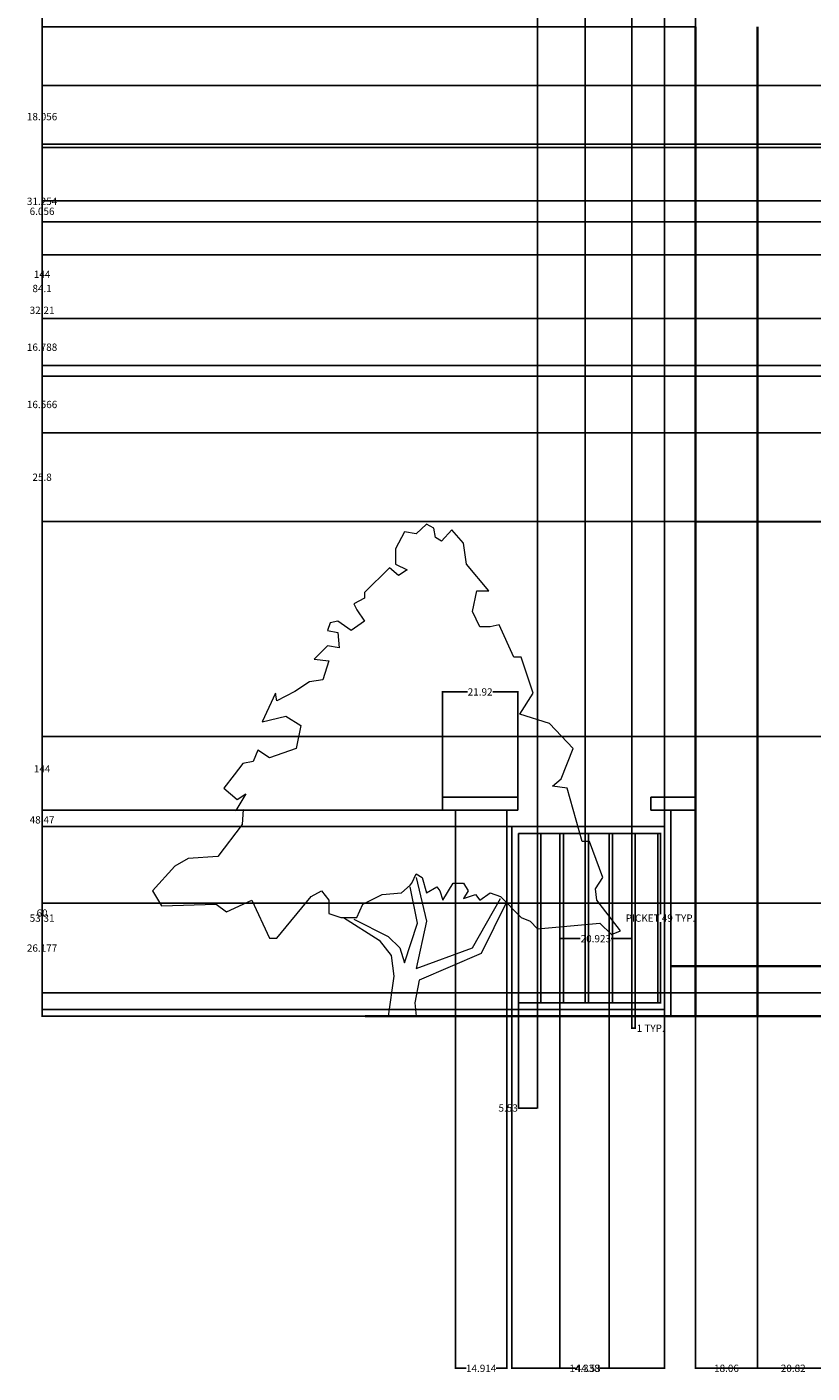
# Model space of a CAD drawing. Units: inches. Extents: x -113 to 379, y 13 to 689.
# Tile 1 of 5: x -113 to 116, y 13 to 405. Entities that reach past the tile are written whole.
import ezdxf

# ---------------------------------------------------------------- set-up
doc = ezdxf.new("R2010")
doc.units = ezdxf.units.IN
doc.header["$MEASUREMENT"] = 0
for name, color, linetype, lineweight in [('A-ANNO-DIMS', 2, 'Continuous', 18), ('A-FLOR', 7, 'Continuous', 30), ('A-WALL', 7, 'Continuous', 35), ('C-TOPO', 8, 'Continuous', 35), ('L-FENC', 8, 'Continuous', 25), ('L-PLNT-TREE', 3, 'Continuous', 13)]:
    doc.layers.add(name, color=color, linetype=linetype, lineweight=lineweight)
doc.styles.get("Standard").update_dxf_attribs({"font": 'arial.ttf'})
doc.dimstyles.get("Standard").update_dxf_attribs({"dimtxt": 2.125, "dimasz": 0.18, "dimexe": 0.18, "dimexo": 0.0625, "dimgap": 0.09, "dimtad": 0, "dimtih": 1, "dimtoh": 1, "dimdec": 4, "dimzin": 0, "dimdsep": 46, "dimlunit": 4, "dimtxsty": 'Standard', "dimcen": 0.09, "dimadec": 0, "dimazin": 0, "dimtfac": 1, "dimtdec": 4, "dimtofl": 0, "dimtmove": 0, "dimatfit": 3, "dimfxl": 1, "dimtolj": 1, "dimtzin": 0, "dimarcsym": 0})

# ---------------------------------------------------------------- blocks, each defined once
blk = doc.blocks.new('*U2')
for points in [[(22.0124, 137.721), (18.5475, 141.5624), (15.5282, 138.2446), (13.8028, 139.3505), (13.3714, 142.1153), (11.2148, 143.2214), (8.1954, 140.4564), (4.7447, 141.0094), (2.1567, 136.0326), (2.1567, 131.6088), (5.6074, 129.9499), (3.0193, 128.2909), (0.4313, 130.5029), (-6.9015, 123.3141), (-6.9015, 121.6552), (-9.9208, 119.9963), (-9.0581, 118.3373), (-6.9015, 115.0195), (-10.7835, 112.2546), (-14.6656, 115.0195), (-16.8222, 114.4665), (-17.6849, 112.2546), (-14.6656, 111.7016), (-14.2342, 107.2778), (-17.6065, 107.8307), (-21.5669, 103.9599), (-17.2536, 103.4069), (-18.9789, 97.8771), (-22.8609, 97.3241), (-27.1743, 94.5593), (-32.3504, 91.7944), (-32.7817, 94.0063), (-36.6638, 85.7116), (-29.7624, 87.3705), (-25.449, 84.6056), (-26.743, 77.9699), (-34.507, 75.205), (-37.9578, 77.4169), (-39.2518, 74.099), (-42.2711, 73.5461), (-44.8592, 70.2282), (-47.8786, 66.3574), (-43.9965, 63.0395), (-41.4085, 64.6985), (-44.3346, 59.8898), (-42.2089, 60.1377), (-42.5159, 55.7849), (-49.6039, 46.4502), (-58.2307, 45.8972), (-62.1127, 43.6853), (-68.5828, 36.4966), (-65.9947, 32.0727), (-50.0352, 32.6257), (-47.0159, 30.4138), (-39.6831, 33.7317), (-34.507, 22.6721), (-32.3504, 22.6721), (-22.4296, 34.8376), (-19.4102, 36.4966), (-17.2536, 33.7317), (-17.2536, 29.8608), (-13.8028, 28.7549), (-9.0581, 28.7549), (-7.3328, 32.6257), (-1.7254, 35.3906), (3.8821, 35.9436), (6.4701, 38.1555), (6.9014, 38.7085), (8.1954, 41.4734), (9.9208, 40.3674), (11.2148, 35.9436), (14.2341, 37.6025), (15.0968, 36.4966), (15.9595, 33.7317), (18.9789, 38.7085), (21.9982, 38.7085), (23.2922, 36.4966), (21.9982, 34.2847), (25.4489, 35.3906), (26.743, 33.7317), (29.7623, 35.9436), (32.7817, 34.8376), (38.8204, 28.7549), (41.4084, 27.6489), (43.5651, 25.437), (61.6813, 27.0959), (65.132, 23.7781), (67.7201, 24.884), (60.8186, 33.7317), (60.3873, 37.0495), (62.544, 40.3674), (58.662, 50.874), (56.5053, 50.874), (52.1919, 66.3574), (47.8785, 66.9103), (50.4665, 69.1222), (53.9172, 77.9699), (47.0158, 85.1586), (38.3891, 87.9235), (42.2711, 94.0063)], [(42.2711, 94.0063), (38.8204, 104.5129), (36.6637, 104.5129), (32.3503, 113.9135), (29.7623, 113.3605), (26.743, 113.3605), (24.5862, 117.7844), (25.8802, 123.8671), (29.331, 123.8671), (22.8609, 131.6088), (21.9982, 137.6916)], [(8.1954, 40.3674), (11.2148, 27.6489), (8.1954, 13.8245), (24.5862, 19.9072), (32.7817, 34.2847)], [(-9.9208, 28.2019), (0, 23.2251), (3.4507, 19.9072), (4.7447, 15.4834), (8.6267, 27.0959), (6.4701, 37.6025)], [(34.5071, 33.1787), (27.1743, 18.2483), (9.0581, 10.5066), (7.7641, 3.8708), (8.1954, 0)], [(-12.9401, 28.7549), (-2.588, 22.1191), (0.8626, 17.6953), (1.7253, 11.6125), (0, 0)]]:
    blk.add_lwpolyline(points)
blk = doc.blocks.new('GATE-PICKET')
for p, q in [((0, 49.31), (0, 0)), ((1, 49.31), (1, 0))]:
    blk.add_line(p, q)
blk = doc.blocks.new('*D9')
at = {"layer": 'A-ANNO-DIMS', "color": 0, "lineweight": -2, "transparency": 16777216}
for p, q in [((64.35, 169.85), (71.87, 169.85)), ((71.69, 169.67), (71.69, 146.38)), ((71.69, 120.72), (71.69, 144)), ((64.35, 120.54), (71.87, 120.54))]:
    blk.add_line(p, q, dxfattribs=at)
at = {"layer": 'A-ANNO-DIMS', "color": 0, "transparency": 16777216}
for points in [[(71.66, 169.67), (71.72, 169.67), (71.69, 169.85)], [(71.66, 120.72), (71.72, 120.72), (71.69, 120.54)]]:
    blk.add_solid(points, dxfattribs=at)
at = {"layer": 'Defpoints', "color": 0, "transparency": 16777216}
for p in [(64.29, 169.85), (71.69, 169.85), (64.29, 120.54)]:
    blk.add_point(p, dxfattribs=at)
at = {"layer": 'A-ANNO-DIMS', "color": 0, "transparency": 16777216, "insert": (71.69, 145.19), "char_height": 2.125, "attachment_point": 5}
blk.add_mtext('\\A1;PICKET 49 TYP.', dxfattribs=at)
blk = doc.blocks.new('*D10')
at = {"layer": 'A-ANNO-DIMS', "color": 0, "lineweight": -2, "transparency": 16777216}
for p, q in [((63.29, 120.48), (63.29, 112.96)), ((64.29, 120.48), (64.29, 112.96)), ((63.47, 113.14), (64.11, 113.14)), ((64.29, 113.14), (64.47, 113.14))]:
    blk.add_line(p, q, dxfattribs=at)
at = {"layer": 'A-ANNO-DIMS', "color": 0, "transparency": 16777216}
for points in [[(63.47, 113.17), (63.47, 113.11), (63.29, 113.14)], [(64.11, 113.17), (64.11, 113.11), (64.29, 113.14)]]:
    blk.add_solid(points, dxfattribs=at)
at = {"layer": 'Defpoints', "color": 0, "transparency": 16777216}
for p in [(63.29, 120.54), (64.29, 120.54), (64.29, 113.14)]:
    blk.add_point(p, dxfattribs=at)
at = {"layer": 'A-ANNO-DIMS', "color": 0, "transparency": 16777216, "insert": (68.81, 113.14), "char_height": 2.125, "attachment_point": 5}
blk.add_mtext('\\A1;1 TYP.', dxfattribs=at)
blk = doc.blocks.new('*D19')
at = {"layer": 'A-ANNO-DIMS', "color": 0, "lineweight": -2, "transparency": 16777216}
for p, q in [((81.87, 116.59), (81.87, 13.95)), ((343.87, 116.59), (343.87, 13.95)), ((82.05, 14.13), (210.43, 14.13)), ((343.69, 14.13), (215.32, 14.13))]:
    blk.add_line(p, q, dxfattribs=at)
at = {"layer": 'A-ANNO-DIMS', "color": 0, "transparency": 16777216}
for points in [[(82.05, 14.16), (82.05, 14.1), (81.87, 14.13)], [(343.69, 14.16), (343.69, 14.1), (343.87, 14.13)]]:
    blk.add_solid(points, dxfattribs=at)
at = {"layer": 'Defpoints', "color": 0, "transparency": 16777216}
for p in [(81.87, 116.65), (343.87, 116.65), (343.87, 14.13)]:
    blk.add_point(p, dxfattribs=at)
at = {"layer": 'A-ANNO-DIMS', "color": 0, "transparency": 16777216, "insert": (212.87, 14.13), "char_height": 2.125, "attachment_point": 5}
blk.add_mtext('\\A1;262', dxfattribs=at)
blk = doc.blocks.new('*D29')
at = {"layer": 'A-ANNO-DIMS', "color": 0, "lineweight": -2, "transparency": 16777216}
for p, q in [((81.81, 548.65), (-108.66, 548.65)), ((-108.48, 548.47), (-108.48, 477.81)), ((-108.48, 404.83), (-108.48, 475.49)), ((81.81, 404.65), (-108.66, 404.65))]:
    blk.add_line(p, q, dxfattribs=at)
at = {"layer": 'A-ANNO-DIMS', "color": 0, "transparency": 16777216}
for points in [[(-108.51, 548.47), (-108.45, 548.47), (-108.48, 548.65)], [(-108.51, 404.83), (-108.45, 404.83), (-108.48, 404.65)]]:
    blk.add_solid(points, dxfattribs=at)
at = {"layer": 'Defpoints', "color": 0, "transparency": 16777216}
for p in [(-108.48, 548.65), (81.87, 548.65), (81.87, 404.65)]:
    blk.add_point(p, dxfattribs=at)
at = {"layer": 'A-ANNO-DIMS', "color": 0, "transparency": 16777216, "insert": (-108.48, 476.65), "char_height": 2.125, "attachment_point": 5}
blk.add_mtext('\\A1;144', dxfattribs=at)
blk = doc.blocks.new('*D30')
at = {"layer": 'A-ANNO-DIMS', "color": 0, "lineweight": -2, "transparency": 16777216}
for p, q in [((81.81, 260.65), (-108.66, 260.65)), ((-108.48, 260.47), (-108.48, 189.81)), ((-108.48, 116.83), (-108.48, 187.49)), ((81.81, 116.65), (-108.66, 116.65))]:
    blk.add_line(p, q, dxfattribs=at)
at = {"layer": 'A-ANNO-DIMS', "color": 0, "transparency": 16777216}
for points in [[(-108.51, 260.47), (-108.45, 260.47), (-108.48, 260.65)], [(-108.51, 116.83), (-108.45, 116.83), (-108.48, 116.65)]]:
    blk.add_solid(points, dxfattribs=at)
at = {"layer": 'Defpoints', "color": 0, "transparency": 16777216}
for p in [(-108.48, 260.65), (81.87, 260.65), (81.87, 116.65)]:
    blk.add_point(p, dxfattribs=at)
at = {"layer": 'A-ANNO-DIMS', "color": 0, "transparency": 16777216, "insert": (-108.48, 188.65), "char_height": 2.125, "attachment_point": 5}
blk.add_mtext('\\A1;144', dxfattribs=at)
blk = doc.blocks.new('*D31')
at = {"layer": 'A-ANNO-DIMS', "color": 0, "lineweight": -2, "transparency": 16777216}
for p, q in [((81.81, 404.65), (-108.66, 404.65)), ((-108.48, 404.47), (-108.48, 333.81)), ((-108.48, 260.83), (-108.48, 331.49)), ((81.81, 260.65), (-108.66, 260.65))]:
    blk.add_line(p, q, dxfattribs=at)
at = {"layer": 'A-ANNO-DIMS', "color": 0, "transparency": 16777216}
for points in [[(-108.51, 404.47), (-108.45, 404.47), (-108.48, 404.65)], [(-108.51, 260.83), (-108.45, 260.83), (-108.48, 260.65)]]:
    blk.add_solid(points, dxfattribs=at)
at = {"layer": 'Defpoints', "color": 0, "transparency": 16777216}
for p in [(-108.48, 404.65), (81.87, 404.65), (81.87, 260.65)]:
    blk.add_point(p, dxfattribs=at)
at = {"layer": 'A-ANNO-DIMS', "color": 0, "transparency": 16777216, "insert": (-108.48, 332.65), "char_height": 2.125, "attachment_point": 5}
blk.add_mtext('\\A1;144', dxfattribs=at)
blk = doc.blocks.new('*D36')
at = {"layer": 'A-ANNO-DIMS', "color": 0, "lineweight": -2, "transparency": 16777216}
for p, q in [((81.87, 116.59), (81.87, 13.95)), ((99.93, 116.59), (99.93, 13.95)), ((82.05, 14.13), (87.33, 14.13)), ((99.75, 14.13), (94.48, 14.13))]:
    blk.add_line(p, q, dxfattribs=at)
at = {"layer": 'A-ANNO-DIMS', "color": 0, "transparency": 16777216}
for points in [[(82.05, 14.16), (82.05, 14.1), (81.87, 14.13)], [(99.75, 14.16), (99.75, 14.1), (99.93, 14.13)]]:
    blk.add_solid(points, dxfattribs=at)
at = {"layer": 'Defpoints', "color": 0, "transparency": 16777216}
for p in [(81.87, 116.65), (99.93, 116.65), (99.93, 14.13)]:
    blk.add_point(p, dxfattribs=at)
at = {"layer": 'A-ANNO-DIMS', "color": 0, "transparency": 16777216, "insert": (90.9, 14.13), "char_height": 2.125, "attachment_point": 5}
blk.add_mtext('\\A1;18.06', dxfattribs=at)
blk = doc.blocks.new('*D37')
at = {"layer": 'A-ANNO-DIMS', "color": 0, "lineweight": -2, "transparency": 16777216}
for p, q in [((99.93, 116.59), (99.93, 13.95)), ((120.75, 116.59), (120.75, 13.95)), ((100.11, 14.13), (106.66, 14.13)), ((120.57, 14.13), (114.03, 14.13))]:
    blk.add_line(p, q, dxfattribs=at)
at = {"layer": 'A-ANNO-DIMS', "color": 0, "transparency": 16777216}
for points in [[(100.11, 14.16), (100.11, 14.1), (99.93, 14.13)], [(120.57, 14.16), (120.57, 14.1), (120.75, 14.13)]]:
    blk.add_solid(points, dxfattribs=at)
at = {"layer": 'Defpoints', "color": 0, "transparency": 16777216}
for p in [(99.93, 116.65), (120.75, 116.65), (120.75, 14.13)]:
    blk.add_point(p, dxfattribs=at)
at = {"layer": 'A-ANNO-DIMS', "color": 0, "transparency": 16777216, "insert": (110.34, 14.13), "char_height": 2.125, "attachment_point": 5}
blk.add_mtext('\\A1;20.82', dxfattribs=at)
blk = doc.blocks.new('*D38')
at = {"layer": 'A-ANNO-DIMS', "color": 0, "lineweight": -2, "transparency": 16777216}
for p, q in [((289.33, 286.45), (-108.66, 286.45)), ((-108.48, 286.27), (-108.48, 274.73)), ((-108.48, 260.83), (-108.48, 272.38)), ((289.33, 260.65), (-108.66, 260.65))]:
    blk.add_line(p, q, dxfattribs=at)
at = {"layer": 'A-ANNO-DIMS', "color": 0, "transparency": 16777216}
for points in [[(-108.51, 286.27), (-108.45, 286.27), (-108.48, 286.45)], [(-108.51, 260.83), (-108.45, 260.83), (-108.48, 260.65)]]:
    blk.add_solid(points, dxfattribs=at)
at = {"layer": 'Defpoints', "color": 0, "transparency": 16777216}
for p in [(-108.48, 286.45), (289.4, 286.45), (289.4, 260.65)]:
    blk.add_point(p, dxfattribs=at)
at = {"layer": 'A-ANNO-DIMS', "color": 0, "transparency": 16777216, "insert": (-108.48, 273.55), "char_height": 2.125, "attachment_point": 5}
blk.add_mtext('\\A1;25.8', dxfattribs=at)
blk = doc.blocks.new('*D40')
at = {"layer": 'A-ANNO-DIMS', "color": 0, "lineweight": -2, "transparency": 16777216}
for p, q in [((145.14, 370.54), (-108.66, 370.54)), ((-108.48, 370.36), (-108.48, 329.67)), ((-108.48, 286.63), (-108.48, 327.32)), ((145.14, 286.45), (-108.66, 286.45))]:
    blk.add_line(p, q, dxfattribs=at)
at = {"layer": 'A-ANNO-DIMS', "color": 0, "transparency": 16777216}
for points in [[(-108.51, 370.36), (-108.45, 370.36), (-108.48, 370.54)], [(-108.51, 286.63), (-108.45, 286.63), (-108.48, 286.45)]]:
    blk.add_solid(points, dxfattribs=at)
at = {"layer": 'Defpoints', "color": 0, "transparency": 16777216}
for p in [(-108.48, 370.54), (145.2, 370.54), (145.2, 286.45)]:
    blk.add_point(p, dxfattribs=at)
at = {"layer": 'A-ANNO-DIMS', "color": 0, "transparency": 16777216, "insert": (-108.48, 328.5), "char_height": 2.125, "attachment_point": 5}
blk.add_mtext('\\A1;84.1', dxfattribs=at)
blk = doc.blocks.new('*D47')
at = {"layer": 'A-ANNO-DIMS', "color": 0, "lineweight": -2, "transparency": 16777216}
for p, q in [((28.33, 118.48), (28.33, 13.95)), ((72.86, 118.48), (72.86, 13.95)), ((28.51, 14.13), (46.88, 14.13)), ((72.68, 14.13), (54.31, 14.13))]:
    blk.add_line(p, q, dxfattribs=at)
at = {"layer": 'A-ANNO-DIMS', "color": 0, "transparency": 16777216}
for points in [[(28.51, 14.16), (28.51, 14.1), (28.33, 14.13)], [(72.68, 14.16), (72.68, 14.1), (72.86, 14.13)]]:
    blk.add_solid(points, dxfattribs=at)
at = {"layer": 'Defpoints', "color": 0, "transparency": 16777216}
for p in [(28.33, 118.54), (72.86, 118.54), (72.86, 14.13)]:
    blk.add_point(p, dxfattribs=at)
at = {"layer": 'A-ANNO-DIMS', "color": 0, "transparency": 16777216, "insert": (50.6, 14.13), "char_height": 2.125, "attachment_point": 5}
blk.add_mtext('\\A1;44.53', dxfattribs=at)
blk = doc.blocks.new('*D48')
at = {"layer": 'A-ANNO-DIMS', "color": 0, "lineweight": -2, "transparency": 16777216}
for p, q in [((28.27, 171.85), (-108.66, 171.85)), ((-108.48, 171.67), (-108.48, 146.37)), ((-108.48, 118.72), (-108.48, 144.02)), ((28.27, 118.54), (-108.66, 118.54))]:
    blk.add_line(p, q, dxfattribs=at)
at = {"layer": 'A-ANNO-DIMS', "color": 0, "transparency": 16777216}
for points in [[(-108.51, 171.67), (-108.45, 171.67), (-108.48, 171.85)], [(-108.51, 118.72), (-108.45, 118.72), (-108.48, 118.54)]]:
    blk.add_solid(points, dxfattribs=at)
at = {"layer": 'Defpoints', "color": 0, "transparency": 16777216}
for p in [(28.33, 171.85), (-108.48, 118.54), (28.33, 118.54)]:
    blk.add_point(p, dxfattribs=at)
at = {"layer": 'A-ANNO-DIMS', "color": 0, "transparency": 16777216, "insert": (-108.48, 145.19), "char_height": 2.125, "attachment_point": 5}
blk.add_mtext('\\A1;53.31', dxfattribs=at)
blk = doc.blocks.new('*D49')
at = {"layer": 'A-ANNO-DIMS', "color": 0, "lineweight": -2, "transparency": 16777216}
for p, q in [((11.97, 116.59), (11.97, 13.95)), ((26.89, 116.59), (26.89, 13.95)), ((12.15, 14.13), (15.03, 14.13)), ((26.71, 14.13), (23.83, 14.13))]:
    blk.add_line(p, q, dxfattribs=at)
at = {"layer": 'A-ANNO-DIMS', "color": 0, "transparency": 16777216}
for points in [[(12.15, 14.16), (12.15, 14.1), (11.97, 14.13)], [(26.71, 14.16), (26.71, 14.1), (26.89, 14.13)]]:
    blk.add_solid(points, dxfattribs=at)
at = {"layer": 'Defpoints', "color": 0, "transparency": 16777216}
for p in [(11.97, 116.65), (26.89, 116.65), (26.89, 14.13)]:
    blk.add_point(p, dxfattribs=at)
at = {"layer": 'A-ANNO-DIMS', "color": 0, "transparency": 16777216, "insert": (19.43, 14.13), "char_height": 2.125, "attachment_point": 5}
blk.add_mtext('\\A1;14.914', dxfattribs=at)
blk = doc.blocks.new('*D50')
at = {"layer": 'A-ANNO-DIMS', "color": 0, "lineweight": -2, "transparency": 16777216}
for p, q in [((72.86, 171.91), (72.86, 688.12)), ((73.04, 687.94), (74.72, 687.94)), ((81.69, 687.94), (80.01, 687.94)), ((81.87, 180.47), (81.87, 688.12))]:
    blk.add_line(p, q, dxfattribs=at)
at = {"layer": 'A-ANNO-DIMS', "color": 0, "transparency": 16777216}
for points in [[(73.04, 687.97), (73.04, 687.91), (72.86, 687.94)], [(81.69, 687.97), (81.69, 687.91), (81.87, 687.94)]]:
    blk.add_solid(points, dxfattribs=at)
at = {"layer": 'Defpoints', "color": 0, "transparency": 16777216}
for p in [(81.87, 687.94), (81.87, 180.4), (72.86, 171.85)]:
    blk.add_point(p, dxfattribs=at)
at = {"layer": 'A-ANNO-DIMS', "color": 0, "transparency": 16777216, "insert": (77.37, 687.94), "char_height": 2.125, "attachment_point": 5}
blk.add_mtext('\\A1;9.01', dxfattribs=at)
blk = doc.blocks.new('*D51')
at = {"layer": 'A-ANNO-DIMS', "color": 0, "lineweight": -2, "transparency": 16777216}
for p, q in [((11.91, 176.65), (-108.66, 176.65)), ((-108.48, 176.47), (-108.48, 147.83)), ((-108.48, 116.83), (-108.48, 145.48)), ((11.91, 116.65), (-108.66, 116.65))]:
    blk.add_line(p, q, dxfattribs=at)
at = {"layer": 'A-ANNO-DIMS', "color": 0, "transparency": 16777216}
for points in [[(-108.51, 176.47), (-108.45, 176.47), (-108.48, 176.65)], [(-108.51, 116.83), (-108.45, 116.83), (-108.48, 116.65)]]:
    blk.add_solid(points, dxfattribs=at)
at = {"layer": 'Defpoints', "color": 0, "transparency": 16777216}
for p in [(-108.48, 176.65), (11.97, 176.65), (11.97, 116.65)]:
    blk.add_point(p, dxfattribs=at)
at = {"layer": 'A-ANNO-DIMS', "color": 0, "transparency": 16777216, "insert": (-108.48, 146.65), "char_height": 2.125, "attachment_point": 5}
blk.add_mtext('\\A1;60', dxfattribs=at)
blk = doc.blocks.new('*D52')
at = {"layer": 'A-ANNO-DIMS', "color": 0, "lineweight": -2, "transparency": 16777216}
for p, q in [((8.17, 180.47), (8.17, 211.22)), ((8.35, 211.04), (15.45, 211.04)), ((29.91, 211.04), (22.81, 211.04)), ((30.09, 180.47), (30.09, 211.22))]:
    blk.add_line(p, q, dxfattribs=at)
at = {"layer": 'A-ANNO-DIMS', "color": 0, "transparency": 16777216}
for points in [[(8.35, 211.07), (8.35, 211.01), (8.17, 211.04)], [(29.91, 211.07), (29.91, 211.01), (30.09, 211.04)]]:
    blk.add_solid(points, dxfattribs=at)
at = {"layer": 'Defpoints', "color": 0, "transparency": 16777216}
for p in [(30.09, 211.04), (8.17, 180.4), (30.09, 180.4)]:
    blk.add_point(p, dxfattribs=at)
at = {"layer": 'A-ANNO-DIMS', "color": 0, "transparency": 16777216, "insert": (19.13, 211.04), "char_height": 2.125, "attachment_point": 5}
blk.add_mtext('\\A1;21.92', dxfattribs=at)
blk = doc.blocks.new('*D53')
at = {"layer": 'A-ANNO-DIMS', "color": 0, "lineweight": -2, "transparency": 16777216}
for p, q in [((125.75, 198.04), (-108.66, 198.04)), ((-108.48, 197.86), (-108.48, 174.97)), ((-108.48, 149.74), (-108.48, 172.62)), ((125.75, 149.56), (-108.66, 149.56))]:
    blk.add_line(p, q, dxfattribs=at)
at = {"layer": 'A-ANNO-DIMS', "color": 0, "transparency": 16777216}
for points in [[(-108.51, 197.86), (-108.45, 197.86), (-108.48, 198.04)], [(-108.51, 149.74), (-108.45, 149.74), (-108.48, 149.56)]]:
    blk.add_solid(points, dxfattribs=at)
at = {"layer": 'Defpoints', "color": 0, "transparency": 16777216}
for p in [(125.81, 198.04), (-108.48, 149.56), (125.81, 149.56)]:
    blk.add_point(p, dxfattribs=at)
at = {"layer": 'A-ANNO-DIMS', "color": 0, "transparency": 16777216, "insert": (-108.48, 173.8), "char_height": 2.125, "attachment_point": 5}
blk.add_mtext('\\A1;48.47', dxfattribs=at)
blk = doc.blocks.new('*D54')
at = {"layer": 'A-ANNO-DIMS', "color": 0, "lineweight": -2, "transparency": 16777216}
for p, q in [((125.75, 149.56), (-108.66, 149.56)), ((-108.48, 149.38), (-108.48, 137.65)), ((-108.48, 123.57), (-108.48, 135.3)), ((125.75, 123.39), (-108.66, 123.39))]:
    blk.add_line(p, q, dxfattribs=at)
at = {"layer": 'A-ANNO-DIMS', "color": 0, "transparency": 16777216}
for points in [[(-108.51, 149.38), (-108.45, 149.38), (-108.48, 149.56)], [(-108.51, 123.57), (-108.45, 123.57), (-108.48, 123.39)]]:
    blk.add_solid(points, dxfattribs=at)
at = {"layer": 'Defpoints', "color": 0, "transparency": 16777216}
for p in [(125.81, 149.56), (-108.48, 123.39), (125.81, 123.39)]:
    blk.add_point(p, dxfattribs=at)
at = {"layer": 'A-ANNO-DIMS', "color": 0, "transparency": 16777216, "insert": (-108.48, 136.47), "char_height": 2.125, "attachment_point": 5}
blk.add_mtext('\\A1;26.177', dxfattribs=at)
blk = doc.blocks.new('*D60')
at = {"layer": 'A-ANNO-DIMS', "color": 0, "lineweight": -2, "transparency": 16777216}
for p, q in [((120.69, 303.02), (-108.66, 303.02)), ((-108.48, 302.84), (-108.48, 295.91)), ((-108.48, 286.63), (-108.48, 293.56)), ((120.69, 286.45), (-108.66, 286.45))]:
    blk.add_line(p, q, dxfattribs=at)
at = {"layer": 'A-ANNO-DIMS', "color": 0, "transparency": 16777216}
for points in [[(-108.51, 302.84), (-108.45, 302.84), (-108.48, 303.02)], [(-108.51, 286.63), (-108.45, 286.63), (-108.48, 286.45)]]:
    blk.add_solid(points, dxfattribs=at)
at = {"layer": 'Defpoints', "color": 0, "transparency": 16777216}
for p in [(-108.48, 303.02), (120.75, 303.02), (120.75, 286.45)]:
    blk.add_point(p, dxfattribs=at)
at = {"layer": 'A-ANNO-DIMS', "color": 0, "transparency": 16777216, "insert": (-108.48, 294.73), "char_height": 2.125, "attachment_point": 5}
blk.add_mtext('\\A1;16.566', dxfattribs=at)
blk = doc.blocks.new('*D61')
at = {"layer": 'A-ANNO-DIMS', "color": 0, "lineweight": -2, "transparency": 16777216}
for p, q in [((120.69, 319.8), (-108.66, 319.8)), ((-108.48, 319.62), (-108.48, 312.58)), ((-108.48, 303.2), (-108.48, 310.23)), ((120.69, 303.02), (-108.66, 303.02))]:
    blk.add_line(p, q, dxfattribs=at)
at = {"layer": 'A-ANNO-DIMS', "color": 0, "transparency": 16777216}
for points in [[(-108.51, 319.62), (-108.45, 319.62), (-108.48, 319.8)], [(-108.51, 303.2), (-108.45, 303.2), (-108.48, 303.02)]]:
    blk.add_solid(points, dxfattribs=at)
at = {"layer": 'Defpoints', "color": 0, "transparency": 16777216}
for p in [(-108.48, 319.8), (120.75, 319.8), (120.75, 303.02)]:
    blk.add_point(p, dxfattribs=at)
at = {"layer": 'A-ANNO-DIMS', "color": 0, "transparency": 16777216, "insert": (-108.48, 311.41), "char_height": 2.125, "attachment_point": 5}
blk.add_mtext('\\A1;16.788', dxfattribs=at)
blk = doc.blocks.new('*D65')
at = {"layer": 'A-ANNO-DIMS', "color": 0, "lineweight": -2, "transparency": 16777216}
for p, q in [((297.67, 338.26), (-108.66, 338.26)), ((-108.48, 338.08), (-108.48, 323.33)), ((-108.48, 306.22), (-108.48, 320.98)), ((297.67, 306.04), (-108.66, 306.04))]:
    blk.add_line(p, q, dxfattribs=at)
at = {"layer": 'A-ANNO-DIMS', "color": 0, "transparency": 16777216}
for points in [[(-108.51, 338.08), (-108.45, 338.08), (-108.48, 338.26)], [(-108.51, 306.22), (-108.45, 306.22), (-108.48, 306.04)]]:
    blk.add_solid(points, dxfattribs=at)
at = {"layer": 'Defpoints', "color": 0, "transparency": 16777216}
for p in [(-108.48, 338.26), (297.73, 338.26), (297.73, 306.04)]:
    blk.add_point(p, dxfattribs=at)
at = {"layer": 'A-ANNO-DIMS', "color": 0, "transparency": 16777216, "insert": (-108.48, 322.15), "char_height": 2.125, "attachment_point": 5}
blk.add_mtext('\\A1;32.21', dxfattribs=at)
blk = doc.blocks.new('*D66')
at = {"layer": 'A-ANNO-DIMS', "color": 0, "lineweight": -2, "transparency": 16777216}
for p, q in [((297.67, 369.51), (-108.66, 369.51)), ((-108.48, 369.33), (-108.48, 355.06)), ((-108.48, 338.44), (-108.48, 352.71)), ((297.67, 338.26), (-108.66, 338.26))]:
    blk.add_line(p, q, dxfattribs=at)
at = {"layer": 'A-ANNO-DIMS', "color": 0, "transparency": 16777216}
for points in [[(-108.51, 369.33), (-108.45, 369.33), (-108.48, 369.51)], [(-108.51, 338.44), (-108.45, 338.44), (-108.48, 338.26)]]:
    blk.add_solid(points, dxfattribs=at)
at = {"layer": 'Defpoints', "color": 0, "transparency": 16777216}
for p in [(-108.48, 369.51), (297.73, 369.51), (297.73, 338.26)]:
    blk.add_point(p, dxfattribs=at)
at = {"layer": 'A-ANNO-DIMS', "color": 0, "transparency": 16777216, "insert": (-108.48, 353.88), "char_height": 2.125, "attachment_point": 5}
blk.add_mtext('\\A1;31.254', dxfattribs=at)
blk = doc.blocks.new('*D67')
at = {"layer": 'A-ANNO-DIMS', "color": 0, "lineweight": -2, "transparency": 16777216}
for p, q in [((297.67, 387.57), (-108.66, 387.57)), ((-108.48, 387.39), (-108.48, 379.71)), ((-108.48, 369.69), (-108.48, 377.36)), ((297.67, 369.51), (-108.66, 369.51))]:
    blk.add_line(p, q, dxfattribs=at)
at = {"layer": 'A-ANNO-DIMS', "color": 0, "transparency": 16777216}
for points in [[(-108.51, 387.39), (-108.45, 387.39), (-108.48, 387.57)], [(-108.51, 369.69), (-108.45, 369.69), (-108.48, 369.51)]]:
    blk.add_solid(points, dxfattribs=at)
at = {"layer": 'Defpoints', "color": 0, "transparency": 16777216}
for p in [(-108.48, 387.57), (297.73, 387.57), (297.73, 369.51)]:
    blk.add_point(p, dxfattribs=at)
at = {"layer": 'A-ANNO-DIMS', "color": 0, "transparency": 16777216, "insert": (-108.48, 378.54), "char_height": 2.125, "attachment_point": 5}
blk.add_mtext('\\A1;18.056', dxfattribs=at)
blk = doc.blocks.new('*D69')
at = {"layer": 'A-ANNO-DIMS', "color": 0, "lineweight": -2, "transparency": 16777216}
for p, q in [((148.49, 353.99), (-108.66, 353.99)), ((-108.48, 353.81), (-108.48, 352.14)), ((-108.48, 348.12), (-108.48, 349.79)), ((148.49, 347.94), (-108.66, 347.94))]:
    blk.add_line(p, q, dxfattribs=at)
at = {"layer": 'A-ANNO-DIMS', "color": 0, "transparency": 16777216}
for points in [[(-108.51, 353.81), (-108.45, 353.81), (-108.48, 353.99)], [(-108.51, 348.12), (-108.45, 348.12), (-108.48, 347.94)]]:
    blk.add_solid(points, dxfattribs=at)
at = {"layer": 'Defpoints', "color": 0, "transparency": 16777216}
for p in [(148.55, 353.99), (-108.48, 347.94), (148.55, 347.94)]:
    blk.add_point(p, dxfattribs=at)
at = {"layer": 'A-ANNO-DIMS', "color": 0, "transparency": 16777216, "insert": (-108.48, 350.97), "char_height": 2.125, "attachment_point": 5}
blk.add_mtext('\\A1;6.056', dxfattribs=at)
blk = doc.blocks.new('*D71')
at = {"layer": 'A-ANNO-DIMS', "color": 0, "lineweight": -2, "transparency": 16777216}
for p, q in [((35.86, 169.91), (35.86, 688.12)), ((36.04, 687.94), (38.39, 687.94)), ((49.55, 687.94), (47.19, 687.94)), ((49.73, 169.91), (49.73, 688.12))]:
    blk.add_line(p, q, dxfattribs=at)
at = {"layer": 'A-ANNO-DIMS', "color": 0, "transparency": 16777216}
for points in [[(36.04, 687.97), (36.04, 687.91), (35.86, 687.94)], [(49.55, 687.97), (49.55, 687.91), (49.73, 687.94)]]:
    blk.add_solid(points, dxfattribs=at)
at = {"layer": 'Defpoints', "color": 0, "transparency": 16777216}
for p in [(49.73, 687.94), (35.86, 169.85), (49.73, 169.85)]:
    blk.add_point(p, dxfattribs=at)
at = {"layer": 'A-ANNO-DIMS', "color": 0, "transparency": 16777216, "insert": (42.79, 687.94), "char_height": 2.125, "attachment_point": 5}
blk.add_mtext('\\A1;13.866', dxfattribs=at)
blk = doc.blocks.new('*D72')
at = {"layer": 'A-ANNO-DIMS', "color": 0, "lineweight": -2, "transparency": 16777216}
for p, q in [((49.73, 169.91), (49.73, 688.12)), ((49.91, 687.94), (52.11, 687.94)), ((63.11, 687.94), (60.91, 687.94)), ((63.29, 169.91), (63.29, 688.12))]:
    blk.add_line(p, q, dxfattribs=at)
at = {"layer": 'A-ANNO-DIMS', "color": 0, "transparency": 16777216}
for points in [[(49.91, 687.97), (49.91, 687.91), (49.73, 687.94)], [(63.11, 687.97), (63.11, 687.91), (63.29, 687.94)]]:
    blk.add_solid(points, dxfattribs=at)
at = {"layer": 'Defpoints', "color": 0, "transparency": 16777216}
for p in [(63.29, 687.94), (49.73, 169.85), (63.29, 169.85)]:
    blk.add_point(p, dxfattribs=at)
at = {"layer": 'A-ANNO-DIMS', "color": 0, "transparency": 16777216, "insert": (56.51, 687.94), "char_height": 2.125, "attachment_point": 5}
blk.add_mtext('\\A1;13.566', dxfattribs=at)
blk = doc.blocks.new('*D73')
at = {"layer": 'A-ANNO-DIMS', "color": 0, "lineweight": -2, "transparency": 16777216}
for p, q in [((42.37, 120.48), (42.37, 13.95)), ((56.71, 120.48), (56.71, 13.95)), ((42.55, 14.13), (45.13, 14.13)), ((56.53, 14.13), (53.94, 14.13))]:
    blk.add_line(p, q, dxfattribs=at)
at = {"layer": 'A-ANNO-DIMS', "color": 0, "transparency": 16777216}
for points in [[(42.55, 14.16), (42.55, 14.1), (42.37, 14.13)], [(56.53, 14.16), (56.53, 14.1), (56.71, 14.13)]]:
    blk.add_solid(points, dxfattribs=at)
at = {"layer": 'Defpoints', "color": 0, "transparency": 16777216}
for p in [(42.37, 120.54), (56.71, 120.54), (56.71, 14.13)]:
    blk.add_point(p, dxfattribs=at)
at = {"layer": 'A-ANNO-DIMS', "color": 0, "transparency": 16777216, "insert": (49.54, 14.13), "char_height": 2.125, "attachment_point": 5}
blk.add_mtext('\\A1;14.338', dxfattribs=at)
blk = doc.blocks.new('*D74')
at = {"layer": 'A-ANNO-DIMS', "color": 0, "lineweight": -2, "transparency": 16777216}
for p, q in [((42.37, 169.78), (42.37, 139.03)), ((63.29, 169.78), (63.29, 139.03)), ((42.55, 139.21), (48.31, 139.21)), ((63.11, 139.21), (57.35, 139.21))]:
    blk.add_line(p, q, dxfattribs=at)
at = {"layer": 'A-ANNO-DIMS', "color": 0, "transparency": 16777216}
for points in [[(42.55, 139.24), (42.55, 139.18), (42.37, 139.21)], [(63.11, 139.24), (63.11, 139.18), (63.29, 139.21)]]:
    blk.add_solid(points, dxfattribs=at)
at = {"layer": 'Defpoints', "color": 0, "transparency": 16777216}
for p in [(42.37, 169.85), (63.29, 169.85), (42.37, 139.21)]:
    blk.add_point(p, dxfattribs=at)
at = {"layer": 'A-ANNO-DIMS', "color": 0, "transparency": 16777216, "insert": (52.83, 139.21), "char_height": 2.125, "attachment_point": 5}
blk.add_mtext('\\A1;20.923', dxfattribs=at)
blk = doc.blocks.new('*D75')
at = {"layer": 'A-ANNO-DIMS', "color": 0, "lineweight": -2, "transparency": 16777216}
for p, q in [((30.33, 120.48), (30.33, 89.72)), ((35.86, 120.48), (35.86, 89.72)), ((30.33, 89.9), (30.15, 89.9)), ((35.68, 89.9), (30.51, 89.9))]:
    blk.add_line(p, q, dxfattribs=at)
at = {"layer": 'A-ANNO-DIMS', "color": 0, "transparency": 16777216}
for points in [[(30.51, 89.93), (30.51, 89.87), (30.33, 89.9)], [(35.68, 89.93), (35.68, 89.87), (35.86, 89.9)]]:
    blk.add_solid(points, dxfattribs=at)
at = {"layer": 'Defpoints', "color": 0, "transparency": 16777216}
for p in [(30.33, 120.54), (35.86, 120.54), (30.33, 89.9)]:
    blk.add_point(p, dxfattribs=at)
at = {"layer": 'A-ANNO-DIMS', "color": 0, "transparency": 16777216, "insert": (27.3, 89.9), "char_height": 2.125, "attachment_point": 5}
blk.add_mtext('\\A1;5.53', dxfattribs=at)

msp = doc.modelspace()

# ---------------------------------------------------------------- linework, layer by layer
at = {"layer": 'A-FLOR'}
msp.add_line((81.8721, 260.6509), (129.5137, 260.6509), dxfattribs=at)
at = {"layer": 'A-WALL'}
for p, q in [((81.8721, 260.6509), (81.8721, 404.6509)), ((99.9328, 260.6509), (99.9328, 404.6509)), ((81.8721, 116.6509), (81.8721, 260.6509)), ((99.9328, 260.6509), (99.9328, 116.6509)), ((74.6887, 131.237), (120.7533, 131.237))]:
    msp.add_line(p, q, dxfattribs=at)
at = {"layer": 'C-TOPO'}
msp.add_line((-14.3304, 116.6509), (343.8693, 116.6509), dxfattribs=at)
at = {"layer": 'L-FENC'}
for p, q in [((8.1694, 176.6509), (8.1694, 180.405)), ((8.1694, 180.405), (30.0916, 180.405)), ((30.0916, 180.405), (30.0916, 176.6509)), ((68.8834, 176.6509), (68.8834, 180.405)), ((68.8834, 180.405), (81.8721, 180.405)), ((11.972, 176.6509), (8.1694, 176.6509)), ((11.972, 116.6509), (11.972, 176.6509)), ((11.972, 176.6509), (26.8857, 176.6509)), ((26.8857, 176.6509), (26.8857, 116.6509)), ((30.0916, 176.6509), (26.8857, 176.6509)), ((70.8236, 176.6509), (68.8834, 176.6509)), ((70.8236, 176.6509), (81.8721, 176.6509)), ((74.6887, 176.6509), (74.6887, 116.6509)), ((74.6887, 176.6509), (81.8721, 176.6509))]:
    msp.add_line(p, q, dxfattribs=at)
for points in [[(28.33, 171.8462), (72.8619, 171.8462), (72.8619, 118.5393), (28.33, 118.5393)], [(30.33, 169.8462), (70.8619, 169.8462), (70.8619, 120.5393), (30.33, 120.5393)]]:
    msp.add_lwpolyline(points, close=True, dxfattribs=at)

# ---------------------------------------------------------------- block references
for p in [(35.86, 120.5393), (42.3686, 120.5393), (49.7256, 120.5393), (56.7062, 120.5393), (63.2917, 120.5393)]:
    msp.add_blockref('GATE-PICKET', p, dxfattribs=at)
at = {"layer": 'L-PLNT-TREE'}
msp.add_blockref('*U2', (-7.6962, 116.6509), dxfattribs=at)

# ---------------------------------------------------------------- dimensions: what is measured, and where the dimension line sits
at = {"layer": 'A-ANNO-DIMS'}
for base, p1, p2, override, picture, middle in [((49.7256, 687.9364), (35.86, 169.8462), (49.7256, 169.8462), {"dimdec": 3, "dimlfac": 1, "dimrnd": 0, "dimzin": 0, "dimdsep": 46, "dimlunit": 2}, '*D71', (42.7928, 687.9364)), ((63.2917, 687.9364), (49.7256, 169.8462), (63.2917, 169.8462), {"dimdec": 3, "dimlfac": 1, "dimrnd": 0, "dimzin": 0, "dimdsep": 46, "dimlunit": 2}, '*D72', (56.5087, 687.9364)), ((81.8721, 687.9364), (72.8619, 171.8462), (81.8721, 180.405), {"dimdec": 2, "dimlfac": 1, "dimrnd": 0, "dimzin": 0, "dimdsep": 46, "dimlunit": 2}, '*D50', (77.367, 687.9364)), ((30.0916, 211.04), (8.1694, 180.405), (30.0916, 180.405), {"dimdec": 2, "dimlfac": 1, "dimrnd": 0, "dimzin": 0, "dimdsep": 46, "dimlunit": 2}, '*D52', (19.1305, 211.04)), ((72.8619, 14.1289), (28.33, 118.5393), (72.8619, 118.5393), {"dimdec": 2, "dimlfac": 1, "dimrnd": 0, "dimzin": 0, "dimdsep": 46, "dimlunit": 2}, '*D47', (50.596, 14.1289)), ((56.7062, 14.1289), (42.3686, 120.5393), (56.7062, 120.5393), {"dimdec": 3, "dimlfac": 1, "dimrnd": 0, "dimzin": 0, "dimdsep": 46, "dimlunit": 2}, '*D73', (49.5374, 14.1289)), ((26.8857, 14.1289), (11.972, 116.6509), (26.8857, 116.6509), {"dimdec": 3, "dimlfac": 1, "dimrnd": 0, "dimzin": 0, "dimdsep": 46, "dimlunit": 2}, '*D49', (19.4288, 14.1289)), ((343.8693, 14.1289), (81.8721, 116.6509), (343.8693, 116.6509), {"dimdec": 0, "dimlfac": 1, "dimrnd": 0, "dimzin": 0, "dimdsep": 46, "dimlunit": 2}, '*D19', (212.8707, 14.1289)), ((99.9328, 14.1289), (81.8721, 116.6509), (99.9328, 116.6509), {"dimdec": 2, "dimlfac": 1, "dimrnd": 0, "dimzin": 0, "dimdsep": 46, "dimlunit": 2}, '*D36', (90.9025, 14.1289)), ((120.7533, 14.1289), (99.9328, 116.6509), (120.7533, 116.6509), {"dimdec": 2, "dimlfac": 1, "dimrnd": 0, "dimzin": 0, "dimdsep": 46, "dimlunit": 2}, '*D37', (110.3431, 14.1289))]:
    dim = msp.add_linear_dim(base=base, p1=p1, p2=p2, dimstyle='Standard', override=override, dxfattribs=at)
    dim.commit()
    dim.dimension.update_dxf_attribs({"geometry": picture, "text_midpoint": middle})
for base, p1, p2, angle, override, picture, middle in [((-108.4772, 548.6509), (81.8721, 404.6509), (81.8721, 548.6509), 90, {"dimdec": 0, "dimlfac": 1, "dimrnd": 0, "dimzin": 0, "dimdsep": 46, "dimlunit": 2}, '*D29', (-108.4772, 476.6509)), ((-108.4772, 404.6509), (81.8721, 260.6509), (81.8721, 404.6509), 90, {"dimdec": 0, "dimlfac": 1, "dimrnd": 0, "dimzin": 0, "dimdsep": 46, "dimlunit": 2}, '*D31', (-108.4772, 332.6509)), ((-108.477185, 387.566634), (297.727979, 369.511131), (297.727979, 387.566634), 90, {"dimdec": 3, "dimlfac": 1, "dimrnd": 0, "dimzin": 0, "dimdsep": 46, "dimlunit": 2}, '*D67', (-108.477185, 378.538882)), ((-108.4772, 369.5111), (297.728, 338.2572), (297.728, 369.5111), 90, {"dimdec": 3, "dimlfac": 1, "dimrnd": 0, "dimzin": 0, "dimdsep": 46, "dimlunit": 2}, '*D66', (-108.4772, 353.8842)), ((-108.4772, 370.5425), (145.1985, 286.4497), (145.1985, 370.5425), 90, {"dimdec": 1, "dimlfac": 1, "dimrnd": 0, "dimzin": 0, "dimdsep": 46, "dimlunit": 2}, '*D40', (-108.4772, 328.4961)), ((-108.4772, 347.9385), (148.5524, 353.9941), (148.5524, 347.9385), 90, {"dimdec": 3, "dimlfac": 1, "dimrnd": 0, "dimzin": 0, "dimdsep": 46, "dimlunit": 2}, '*D69', (-108.4772, 350.9663)), ((-108.4772, 338.2572), (297.728, 306.0445), (297.728, 338.2572), 90, {"dimdec": 2, "dimlfac": 1, "dimrnd": 0, "dimzin": 0, "dimdsep": 46, "dimlunit": 2}, '*D65', (-108.4772, 322.1509)), ((-108.47719, 319.8035), (120.75329, 303.01598), (120.75329, 319.8035), 90, {"dimdec": 3, "dimlfac": 1, "dimrnd": 0, "dimzin": 0, "dimdsep": 46, "dimlunit": 2}, '*D61', (-108.47719, 311.40974)), ((-108.4772, 303.016), (120.7533, 286.4497), (120.7533, 303.016), 90, {"dimdec": 3, "dimlfac": 1, "dimrnd": 0, "dimzin": 0, "dimdsep": 46, "dimlunit": 2}, '*D60', (-108.4772, 294.7329)), ((-108.4772, 286.4497), (289.3958, 260.6509), (289.3958, 286.4497), 90, {"dimdec": 1, "dimlfac": 1, "dimrnd": 0, "dimzin": 0, "dimdsep": 46, "dimlunit": 2}, '*D38', (-108.4772, 273.5503)), ((-108.4772, 260.6509), (81.8721, 116.6509), (81.8721, 260.6509), 90, {"dimdec": 0, "dimlfac": 1, "dimrnd": 0, "dimzin": 0, "dimdsep": 46, "dimlunit": 2}, '*D30', (-108.4772, 188.6509)), ((-108.4772, 149.5623), (125.8084, 198.0351), (125.8084, 149.5623), 90, {"dimdec": 2, "dimlfac": 1, "dimrnd": 0, "dimzin": 0, "dimdsep": 46, "dimlunit": 2}, '*D53', (-108.4772, 173.7987)), ((-108.4772, 176.6509), (11.972, 116.6509), (11.972, 176.6509), 90, {"dimdec": 0, "dimlfac": 1, "dimrnd": 0, "dimzin": 0, "dimdsep": 46, "dimlunit": 2}, '*D51', (-108.4772, 146.6509)), ((-108.4772, 118.5393), (28.33, 171.8462), (28.33, 118.5393), 90, {"dimdec": 2, "dimlfac": 1, "dimrnd": 0, "dimzin": 0, "dimdsep": 46, "dimlunit": 2}, '*D48', (-108.4772, 145.1928)), ((42.3686, 139.2112), (63.2917, 169.8462), (42.3686, 169.8462), 180, {"dimdec": 3, "dimlfac": 1, "dimrnd": 0, "dimzin": 0, "dimdsep": 46, "dimlunit": 2}, '*D74', (52.8301, 139.2112)), ((-108.4772, 123.3856), (125.8084, 149.5623), (125.8084, 123.3856), 90, {"dimdec": 3, "dimlfac": 1, "dimrnd": 0, "dimzin": 0, "dimdsep": 46, "dimlunit": 2}, '*D54', (-108.4772, 136.4739)), ((30.33, 89.9043), (35.86, 120.5393), (30.33, 120.5393), 180, {"dimdec": 2, "dimlfac": 1, "dimrnd": 0, "dimzin": 0, "dimdsep": 46, "dimlunit": 2}, '*D75', (27.3002, 89.9043))]:
    dim = msp.add_linear_dim(base=base, p1=p1, p2=p2, angle=angle, dimstyle='Standard', override=override, dxfattribs=at)
    dim.commit()
    dim.dimension.update_dxf_attribs({"geometry": picture, "text_midpoint": middle})
dim = msp.add_linear_dim(base=(71.6878, 169.8462), p1=(64.2917, 120.5393), p2=(64.2917, 169.8462), angle=90, text='PICKET <> TYP.', dimstyle='Standard', override={"dimdec": 0, "dimlfac": 1, "dimrnd": 0, "dimzin": 0, "dimdsep": 46, "dimlunit": 2}, dxfattribs=at)
dim.commit()
dim.dimension.update_dxf_attribs({"geometry": '*D9', "text_midpoint": (71.6878, 145.1928)})
dim = msp.add_linear_dim(base=(64.2917, 113.1433), p1=(63.2917, 120.5393), p2=(64.2917, 120.5393), text='<> TYP.', dimstyle='Standard', override={"dimdec": 0, "dimlfac": 1, "dimrnd": 0, "dimzin": 0, "dimdsep": 46, "dimlunit": 2}, dxfattribs=at)
dim.commit()
dim.dimension.update_dxf_attribs({"geometry": '*D10', "text_midpoint": (68.8081, 113.1433)})

doc.saveas('drawing.dxf')
